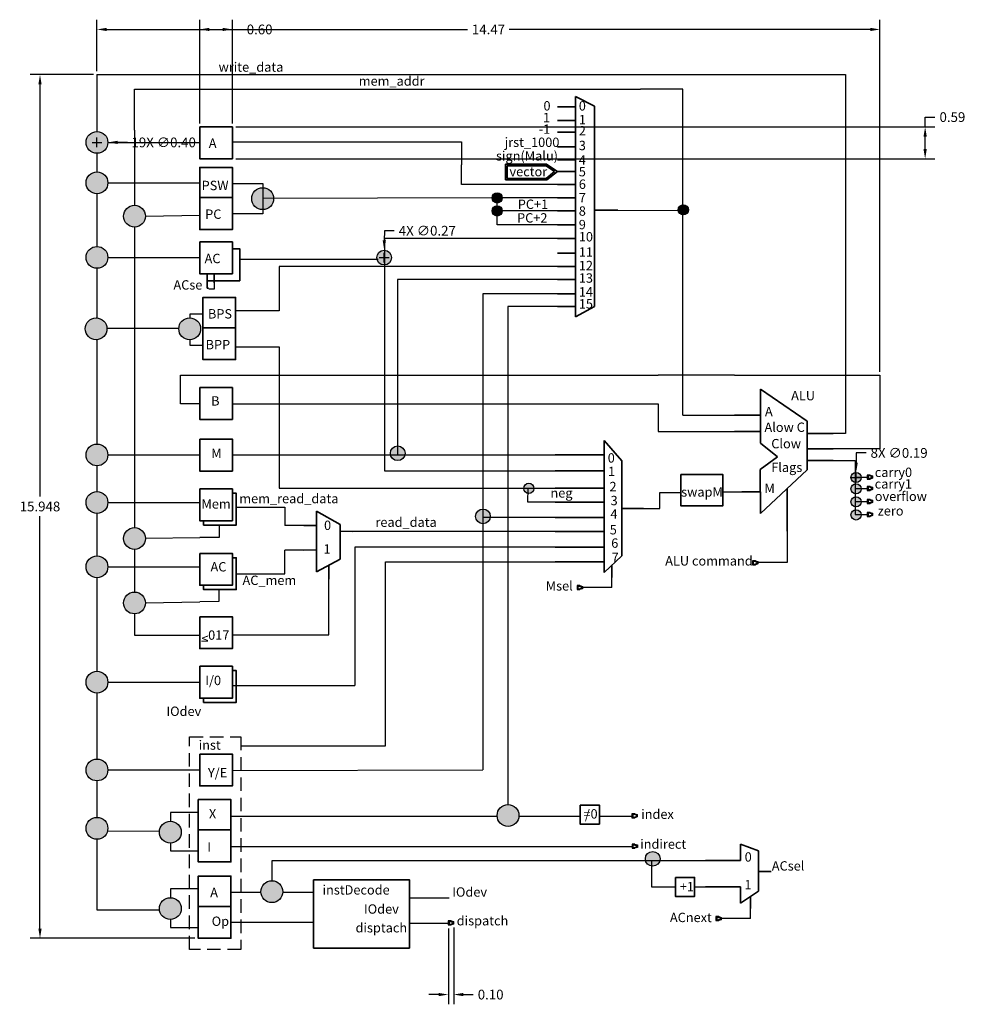
# Model space of a CAD drawing. Units: inches. Extents: x 90.6 to 108.1, y 86.4 to 104.6.
import ezdxf

# ---------------------------------------------------------------- set-up
doc = ezdxf.new("R2010")
doc.units = ezdxf.units.IN
doc.header["$MEASUREMENT"] = 0
doc.linetypes.add('HIDDEN', pattern=[0.375, 0.25, -0.125])
for name, color, linetype, lineweight in [('A-ANNO-DIMS', 2, 'Continuous', 18), ('E-COMP', 1, 'Continuous', 35), ('E-COMP-HIDN', 5, 'HIDDEN', 25), ('E-SYMB', 3, 'Continuous', 25), ('E-TEXT', 4, 'Continuous', 18), ('E-WIRE', 3, 'Continuous', 25)]:
    doc.layers.add(name, color=color, linetype=linetype, lineweight=lineweight)
doc.styles.get("Standard").update_dxf_attribs({"font": 'arial.ttf'})
doc.dimstyles.get("Standard").update_dxf_attribs({"dimtxt": 0.18, "dimasz": 0.18, "dimexe": 0.18, "dimexo": 0.0625, "dimgap": 0.09, "dimtad": 0, "dimtih": 1, "dimtoh": 1, "dimdec": 4, "dimzin": 0, "dimdsep": 46, "dimtxsty": 'Standard', "dimcen": 0.09, "dimadec": 0, "dimazin": 0, "dimtfac": 1, "dimtdec": 4, "dimtofl": 0, "dimtmove": 0, "dimatfit": 3, "dimfxl": 1, "dimtolj": 1, "dimtzin": 0, "dimarcsym": 0})

# ---------------------------------------------------------------- blocks, each defined once
blk = doc.blocks.new('PORT-CONNECTOR')
h = blk.add_hatch(color=256)
h.dxf.hatch_style = 1
h.paths.add_polyline_path([(102.004, 89.371), (101.949, 89.371), (101.949, 89.296), (102.004, 89.296), (102.048, 89.313), (102.048, 89.357), (102.004, 89.371), (102.001, 89.356), (102.033, 89.346), (102.033, 89.323), (102.001, 89.311), (101.965, 89.311), (101.965, 89.356), (102.001, 89.356)])
for p, q in [((101.949, 89.371), (101.949, 89.296)), ((102.004, 89.371), (101.949, 89.371)), ((101.949, 89.296), (102.004, 89.296)), ((101.965, 89.356), (101.965, 89.311)), ((102.001, 89.356), (101.965, 89.356)), ((101.965, 89.311), (102.001, 89.311)), ((102.001, 89.356), (102.033, 89.346)), ((102.033, 89.323), (102.001, 89.311)), ((102.004, 89.371), (102.048, 89.357)), ((102.048, 89.313), (102.004, 89.296)), ((102.033, 89.346), (102.033, 89.323)), ((102.048, 89.357), (102.048, 89.313))]:
    blk.add_line(p, q)
blk = doc.blocks.new('*D2')
at = {"layer": 'A-ANNO-DIMS', "color": 0, "lineweight": -2, "transparency": 16777216}
for p, q in [((92.062, 103.644), (92.062, 104.597)), ((106.531, 98.095), (106.531, 104.597)), ((92.242, 104.417), (98.911, 104.417)), ((106.351, 104.417), (99.682, 104.417))]:
    blk.add_line(p, q, dxfattribs=at)
at = {"layer": 'A-ANNO-DIMS', "color": 0, "transparency": 16777216}
for points in [[(92.242, 104.447), (92.242, 104.387), (92.062, 104.417)], [(106.351, 104.447), (106.351, 104.387), (106.531, 104.417)]]:
    blk.add_solid(points, dxfattribs=at)
at = {"layer": 'Defpoints', "color": 0, "transparency": 16777216}
for p in [(106.531, 104.417), (92.062, 103.582), (106.531, 98.032)]:
    blk.add_point(p, dxfattribs=at)
at = {"layer": 'A-ANNO-DIMS', "color": 0, "transparency": 16777216, "insert": (99.297, 104.417), "char_height": 0.18, "attachment_point": 5}
blk.add_mtext('\\A1;14.47', dxfattribs=at)
blk = doc.blocks.new('*D3')
at = {"layer": 'A-ANNO-DIMS', "color": 0, "lineweight": -2, "transparency": 16777216}
for p, q in [((92, 103.582), (90.829, 103.582)), ((91.009, 103.402), (91.009, 95.79)), ((91.009, 87.814), (91.009, 95.426)), ((93.873, 87.634), (90.829, 87.634))]:
    blk.add_line(p, q, dxfattribs=at)
at = {"layer": 'A-ANNO-DIMS', "color": 0, "transparency": 16777216}
for points in [[(90.979, 103.402), (91.039, 103.402), (91.009, 103.582)], [(90.979, 87.814), (91.039, 87.814), (91.009, 87.634)]]:
    blk.add_solid(points, dxfattribs=at)
at = {"layer": 'Defpoints', "color": 0, "transparency": 16777216}
for p in [(92.062, 103.582), (91.009, 87.634), (93.935, 87.634)]:
    blk.add_point(p, dxfattribs=at)
at = {"layer": 'A-ANNO-DIMS', "color": 0, "transparency": 16777216, "insert": (91.009, 95.608), "char_height": 0.18, "attachment_point": 5}
blk.add_mtext('\\A1;15.948', dxfattribs=at)
blk = doc.blocks.new('*D4')
at = {"layer": 'A-ANNO-DIMS', "color": 0, "lineweight": -2, "transparency": 16777216}
for p, q in [((93.961, 102.68), (93.961, 104.597)), ((94.564, 102.68), (94.564, 104.597)), ((94.141, 104.417), (94.384, 104.417)), ((94.564, 104.417), (94.744, 104.417))]:
    blk.add_line(p, q, dxfattribs=at)
at = {"layer": 'A-ANNO-DIMS', "color": 0, "transparency": 16777216}
for points in [[(94.141, 104.447), (94.141, 104.387), (93.961, 104.417)], [(94.384, 104.447), (94.384, 104.387), (94.564, 104.417)]]:
    blk.add_solid(points, dxfattribs=at)
at = {"layer": 'Defpoints', "color": 0, "transparency": 16777216}
for p in [(94.564, 104.417), (93.961, 102.618), (94.564, 102.618)]:
    blk.add_point(p, dxfattribs=at)
at = {"layer": 'A-ANNO-DIMS', "color": 0, "transparency": 16777216, "insert": (95.068, 104.417), "char_height": 0.18, "attachment_point": 5}
blk.add_mtext('\\A1;0.60', dxfattribs=at)
blk = doc.blocks.new('*D5')
at = {"layer": 'A-ANNO-DIMS', "color": 0, "lineweight": -2, "transparency": 16777216}
for p, q in [((107.366, 102.618), (107.366, 102.798)), ((107.366, 102.798), (107.546, 102.798)), ((94.627, 102.618), (107.546, 102.618)), ((107.366, 102.208), (107.366, 102.438)), ((94.627, 102.028), (107.546, 102.028))]:
    blk.add_line(p, q, dxfattribs=at)
at = {"layer": 'A-ANNO-DIMS', "color": 0, "transparency": 16777216}
for points in [[(107.336, 102.438), (107.396, 102.438), (107.366, 102.618)], [(107.336, 102.208), (107.396, 102.208), (107.366, 102.028)]]:
    blk.add_solid(points, dxfattribs=at)
at = {"layer": 'Defpoints', "color": 0, "transparency": 16777216}
for p in [(94.564, 102.618), (107.366, 102.618), (94.564, 102.028)]:
    blk.add_point(p, dxfattribs=at)
at = {"layer": 'A-ANNO-DIMS', "color": 0, "transparency": 16777216, "insert": (107.87, 102.798), "char_height": 0.18, "attachment_point": 5}
blk.add_mtext('\\A1;0.59', dxfattribs=at)
blk = doc.blocks.new('*D6')
at = {"layer": 'A-ANNO-DIMS', "color": 0, "lineweight": -2, "transparency": 16777216}
for p, q in [((98.654, 87.835), (98.654, 86.415)), ((98.555, 87.818), (98.555, 86.415)), ((98.375, 86.595), (98.195, 86.595)), ((98.834, 86.595), (99.014, 86.595))]:
    blk.add_line(p, q, dxfattribs=at)
at = {"layer": 'A-ANNO-DIMS', "color": 0, "transparency": 16777216}
for points in [[(98.375, 86.625), (98.375, 86.565), (98.555, 86.595)], [(98.834, 86.625), (98.834, 86.565), (98.654, 86.595)]]:
    blk.add_solid(points, dxfattribs=at)
at = {"layer": 'Defpoints', "color": 0, "transparency": 16777216}
for p in [(98.555, 87.88), (98.654, 87.897), (98.654, 86.595)]:
    blk.add_point(p, dxfattribs=at)
at = {"layer": 'A-ANNO-DIMS', "color": 0, "transparency": 16777216, "insert": (99.337, 86.595), "char_height": 0.18, "attachment_point": 5}
blk.add_mtext('\\A1;0.10', dxfattribs=at)
blk = doc.blocks.new('*D7')
at = {"layer": 'A-ANNO-DIMS', "color": 0, "lineweight": -2, "transparency": 16777216}
for p, q in [((92.062, 102.241), (92.062, 102.421)), ((91.972, 102.331), (92.152, 102.331)), ((92.624, 102.331), (92.444, 102.331))]:
    blk.add_line(p, q, dxfattribs=at)
at = {"layer": 'A-ANNO-DIMS', "color": 0, "transparency": 16777216}
blk.add_solid([(92.444, 102.361), (92.444, 102.301), (92.264, 102.331)], dxfattribs=at)
at = {"layer": 'Defpoints', "color": 0, "transparency": 16777216}
for p in [(91.86, 102.331), (92.264, 102.331)]:
    blk.add_point(p, dxfattribs=at)
at = {"layer": 'A-ANNO-DIMS', "color": 0, "transparency": 16777216, "insert": (93.295, 102.331), "char_height": 0.18, "attachment_point": 5}
blk.add_mtext('\\A1;19X ∅0.40', dxfattribs=at)
blk = doc.blocks.new('*D8')
at = {"layer": 'A-ANNO-DIMS', "color": 0, "lineweight": -2, "transparency": 16777216}
for p, q in [((97.374, 100.7), (97.372, 100.52)), ((97.554, 100.7), (97.374, 100.7)), ((97.279, 100.204), (97.459, 100.204)), ((97.369, 100.114), (97.369, 100.294))]:
    blk.add_line(p, q, dxfattribs=at)
at = {"layer": 'A-ANNO-DIMS', "color": 0, "transparency": 16777216}
blk.add_solid([(97.342, 100.521), (97.402, 100.52), (97.37, 100.34)], dxfattribs=at)
at = {"layer": 'Defpoints', "color": 0, "transparency": 16777216}
for p in [(97.37, 100.34), (97.367, 100.068)]:
    blk.add_point(p, dxfattribs=at)
at = {"layer": 'A-ANNO-DIMS', "color": 0, "transparency": 16777216, "insert": (98.167, 100.7), "char_height": 0.18, "attachment_point": 5}
blk.add_mtext('\\A1;4X ∅0.27', dxfattribs=at)
blk = doc.blocks.new('*D9')
at = {"layer": 'A-ANNO-DIMS', "color": 0, "lineweight": -2, "transparency": 16777216}
for p, q in [((106.094, 96.597), (106.092, 96.417)), ((106.274, 96.597), (106.094, 96.597)), ((106.089, 96.053), (106.089, 96.233)), ((105.999, 96.143), (106.179, 96.143))]:
    blk.add_line(p, q, dxfattribs=at)
at = {"layer": 'A-ANNO-DIMS', "color": 0, "transparency": 16777216}
blk.add_solid([(106.062, 96.417), (106.122, 96.417), (106.09, 96.237)], dxfattribs=at)
at = {"layer": 'Defpoints', "color": 0, "transparency": 16777216}
for p in [(106.09, 96.237), (106.088, 96.049)]:
    blk.add_point(p, dxfattribs=at)
at = {"layer": 'A-ANNO-DIMS', "color": 0, "transparency": 16777216, "insert": (106.885, 96.597), "char_height": 0.18, "attachment_point": 5}
blk.add_mtext('\\A1;8X ∅0.19', dxfattribs=at)

msp = doc.modelspace()

# ---------------------------------------------------------------- hatches: boundary and pattern name
at = {"layer": 'E-COMP'}
h = msp.add_hatch(color=256, dxfattribs=at)
h.dxf.hatch_style = 1
h.paths.add_polyline_path([(99.6422, 101.9276), (99.6122, 101.9276), (99.6122, 101.8976), (99.6122, 101.6671), (99.6122, 101.6371), (99.6422, 101.6371), (99.6422, 101.6671)])
h.paths.add_polyline_path([(100.3621, 101.6671), (99.6422, 101.6671), (99.6422, 101.6371), (100.3621, 101.6371)])
h.paths.add_polyline_path([(100.3621, 101.9276), (99.6422, 101.9276), (99.6422, 101.8976), (100.3621, 101.8976)])
h.paths.add_polyline_path([(100.3713, 101.9276), (100.3621, 101.9276), (100.3621, 101.8976), (100.5192, 101.7913), (100.5676, 101.7913), (100.57, 101.7932)])
h.paths.add_polyline_path([(100.5676, 101.7913), (100.5192, 101.7913), (100.3621, 101.6671), (100.3621, 101.6371), (100.3726, 101.6371)])
at = {"layer": 'E-SYMB'}
h = msp.add_hatch(color=256, dxfattribs=at)
h.dxf.hatch_style = 1
h.paths.add_polyline_path([(106.0735, 96.2356, 0.366956), (105.9948, 96.1428, 0.366956), (106.0735, 96.05)])
h.paths.add_polyline_path([(106.0735, 96.2356), (106.0735, 96.1478), (106.1828, 96.1478, 0.4472138)])
h.paths.add_polyline_path([(106.183, 96.1428, 0.0131646), (106.1828, 96.1478), (106.0735, 96.1478), (106.0735, 96.05, 0.4631049)])
h.paths.add_polyline_path([(106.0735, 96.0262), (106.0735, 95.9383), (106.1828, 95.9383, 0.4472138)])
h.paths.add_polyline_path([(106.183, 95.9334, 0.0131646), (106.1828, 95.9383), (106.0735, 95.9383), (106.0735, 95.8405, 0.4631049)])
h.paths.add_polyline_path([(106.0735, 95.9383), (106.0735, 96.0262, 0.366956), (105.9948, 95.9334, 0.366956), (106.0735, 95.8405)])
h.paths.add_polyline_path([(106.0735, 95.7855, 0.366956), (105.9948, 95.6927, 0.366956), (106.0735, 95.5999)])
h.paths.add_polyline_path([(106.0735, 95.7855), (106.0735, 95.6976), (106.1828, 95.6976, 0.4472138)])
h.paths.add_polyline_path([(106.183, 95.6927, 0.0131646), (106.1828, 95.6976), (106.0735, 95.6976), (106.0735, 95.5999, 0.4631049)])
h.paths.add_polyline_path([(106.0735, 95.5448, 0.366956), (105.9948, 95.452, 1), (106.183, 95.452, 0.0131646), (106.1828, 95.4569), (106.0735, 95.4569)])
h.paths.add_polyline_path([(106.0735, 95.5448), (106.0735, 95.4569), (106.1828, 95.4569, 0.4472138)])
h.paths.add_polyline_path([(100.138, 95.9425, 0.0131646), (100.1379, 95.9475), (100.0286, 95.9475), (100.0266, 95.85, 0.4696785)])
h.paths.add_polyline_path([(100.0286, 95.9475), (99.95, 95.9475, 0.0131646), (99.9499, 95.9425, 0.3608418), (100.0266, 95.85)])
h.paths.add_polyline_path([(99.95, 95.9475), (100.0286, 95.9475), (100.1379, 95.9475, 0.9486838)])
h.paths.add_polyline_path([(99.4565, 89.9015, 1), (99.8599, 89.9015, 1)])
h.paths.add_polyline_path([(95.0927, 88.495, 1), (95.4961, 88.495, 1)])
h.paths.add_polyline_path([(93.2164, 88.1826, 1), (93.6198, 88.1826, 1)])
h.paths.add_polyline_path([(93.6198, 89.5947, 1), (93.2164, 89.5947, 1)])
h.paths.add_polyline_path([(92.2638, 89.6647, 1), (91.8604, 89.6647, 1)])
h.paths.add_polyline_path([(91.8604, 90.7425, 1), (92.2638, 90.7425, 1)])
h.paths.add_polyline_path([(92.2638, 92.3637, 1), (91.8604, 92.3637, 1)])
h.paths.add_polyline_path([(92.9584, 93.8266, 1), (92.555, 93.8266, 1)])
h.paths.add_polyline_path([(92.2638, 94.4942, 1), (91.8604, 94.4942, 1)])
h.paths.add_polyline_path([(92.555, 95.0169, 1), (92.9584, 95.0169, 1)])
h.paths.add_polyline_path([(91.8604, 95.6825, 1), (92.2638, 95.6825, 1)])
h.paths.add_polyline_path([(91.8604, 96.5597, 1), (92.2638, 96.5597, 1)])
h.paths.add_polyline_path([(91.8437, 98.8894, 1), (92.247, 98.8894, 1)])
h.paths.add_polyline_path([(93.5739, 98.8894, 1), (93.9773, 98.8894, 1)])
h.paths.add_polyline_path([(91.8604, 100.2075, 1), (92.2638, 100.2075, 1)])
h.paths.add_polyline_path([(92.555, 100.9676, 1), (92.9584, 100.9676, 1)])
h.paths.add_polyline_path([(91.8604, 101.5837, 1), (92.2638, 101.5837, 1)])
h.paths.add_polyline_path([(92.2638, 102.3309, 1), (91.8604, 102.3309, 1)])
h = msp.add_hatch(color=256, dxfattribs=at)
h.dxf.hatch_style = 1
h.paths.add_polyline_path([(95.1242, 101.09, 0.4142136), (95.3259, 101.2917, 0.4142136), (95.1242, 101.4934)])
h.paths.add_polyline_path([(94.9225, 101.2917, 0.4142136), (95.1242, 101.09), (95.1242, 101.4934, 0.4142136)])
h = msp.add_hatch(color=256, dxfattribs=at)
h.dxf.hatch_style = 1
h.paths.add_polyline_path([(99.5508, 101.3059, 1), (99.3627, 101.3059, 1)])
h = msp.add_hatch(color=256, dxfattribs=at)
h.dxf.hatch_style = 1
h.paths.add_polyline_path([(99.4567, 101.1597, 0.4144064), (99.3626, 101.0656, 0.4143029), (99.4567, 100.9715)])
h.paths.add_polyline_path([(99.5507, 101.0656), (99.4567, 101.0656), (99.4567, 100.9715, 0.4141242)])
h.paths.add_polyline_path([(99.4567, 101.1597), (99.4567, 101.0656), (99.5507, 101.0656, 0.4140208)])
h = msp.add_hatch(color=256, dxfattribs=at)
h.dxf.hatch_style = 1
h.paths.add_polyline_path([(102.8877, 101.1789, 0.3829883), (102.8038, 101.0853, 0.3829883), (102.8877, 100.9918)])
h.paths.add_polyline_path([(102.8877, 101.1789), (102.8877, 100.9918, 0.4461438), (102.9919, 101.0853, 0.4461438)])
h = msp.add_hatch(color=256, dxfattribs=at)
h.dxf.hatch_style = 1
h.paths.add_polyline_path([(97.5049, 100.2039, 1), (97.2324, 100.2039, 1)])
h = msp.add_hatch(color=256, dxfattribs=at)
h.dxf.hatch_style = 1
h.paths.add_polyline_path([(97.7557, 96.5908, 1), (97.4832, 96.5908, 1)])
h = msp.add_hatch(color=256, dxfattribs=at)
h.dxf.hatch_style = 1
h.paths.add_polyline_path([(99.3309, 95.4246, 1), (99.0583, 95.4246, 1)])
h = msp.add_hatch(color=256, dxfattribs=at)
h.dxf.hatch_style = 1
h.paths.add_polyline_path([(102.4683, 89.1009, 1), (102.1957, 89.1009, 1)])

# ---------------------------------------------------------------- linework, layer by layer
at = {"layer": 'E-COMP'}
for p, q in [((100.9022, 103.1788), (100.9022, 99.1114)), ((101.2566, 102.9982), (100.9022, 103.1788)), ((100.9022, 102.9879), (100.57, 102.9879)), ((101.2566, 102.8182), (101.2566, 102.9982)), ((100.9022, 102.7363), (100.57, 102.7363)), ((101.2566, 102.8182), (101.2566, 99.2988)), ((100.9022, 102.5213), (100.57, 102.5213)), ((100.9022, 102.2463), (100.57, 102.2463)), ((100.9022, 102.0082), (100.57, 102.0082)), ((99.6122, 101.9276), (100.3621, 101.9276)), ((99.6122, 101.8976), (99.6122, 101.9276)), ((99.6122, 101.8976), (99.6122, 101.6671)), ((99.6422, 101.8976), (100.3621, 101.8976)), ((99.6422, 101.8976), (99.6422, 101.6671)), ((99.6422, 101.8976), (99.6422, 101.6671)), ((100.2827, 101.9845), (100.2827, 101.9845)), ((100.3621, 101.9276), (100.3713, 101.9276)), ((100.5192, 101.7913), (100.3621, 101.8976)), ((100.57, 101.7932), (100.3713, 101.9276)), ((99.6122, 101.6671), (99.6122, 101.6371)), ((99.6122, 101.6371), (100.3621, 101.6371)), ((99.6422, 101.6671), (100.3621, 101.6671)), ((100.3621, 101.6671), (100.5192, 101.7913)), ((100.3621, 101.6371), (100.3726, 101.6371)), ((100.3726, 101.6371), (100.57, 101.7932)), ((100.9022, 101.7932), (100.57, 101.7932)), ((100.9022, 101.5554), (100.57, 101.5554)), ((94.564, 101.3106), (93.9606, 101.3106)), ((100.9022, 101.308), (100.57, 101.308)), ((100.9022, 101.0656), (100.57, 101.0656)), ((101.2566, 101.0774), (101.6846, 101.0774)), ((100.9022, 100.8089), (100.57, 100.8089)), ((100.9022, 100.5569), (100.57, 100.5569)), ((100.9022, 100.287), (100.57, 100.287)), ((100.9022, 100.0395), (100.57, 100.0395)), ((94.2271, 99.9048), (94.2271, 99.7376)), ((94.0975, 99.7767), (94.0975, 99.6376)), ((94.0975, 99.6376), (94.1227, 99.6376)), ((100.9022, 99.8017), (100.57, 99.8017)), ((100.9022, 99.5359), (100.57, 99.5359)), ((100.9022, 99.3027), (100.57, 99.3027)), ((101.2566, 99.2988), (100.9022, 99.1114)), ((94.6224, 98.9092), (94.019, 98.9092)), ((104.3231, 96.7766), (104.3231, 97.7766)), ((104.3231, 97.7766), (105.1867, 97.1862)), ((103.8454, 97.2961), (104.3231, 97.2961)), ((105.1867, 97.1862), (105.1867, 96.2862)), ((103.8454, 96.9943), (104.3231, 96.9943)), ((105.6692, 96.9538), (105.1867, 96.9538)), ((101.4328, 96.8253), (101.4328, 94.3862)), ((101.4328, 96.8253), (101.763, 96.4499)), ((104.3231, 96.7766), (104.6361, 96.5275)), ((100.5301, 96.5597), (101.4328, 96.5597)), ((105.6692, 96.6702), (105.1867, 96.6702)), ((101.763, 96.4499), (101.763, 94.6945)), ((104.6361, 96.5275), (104.3151, 96.2888)), ((105.6692, 96.456), (105.1867, 96.456)), ((100.5301, 96.2671), (101.4328, 96.2671)), ((104.3151, 96.2888), (104.3231, 95.4807)), ((104.3231, 95.4807), (105.1867, 96.2862)), ((100.5301, 95.9475), (101.4328, 95.9475)), ((103.9768, 95.8772), (104.3192, 95.8772)), ((104.8174, 95.9418), (104.8174, 95.1508)), ((100.5301, 95.6867), (101.4328, 95.6867)), ((96.1184, 95.5225), (96.1184, 94.399)), ((96.1184, 95.5225), (96.5539, 95.2768)), ((101.763, 95.5677), (102.163, 95.5677)), ((96.5539, 95.2768), (96.5539, 94.637)), ((100.5301, 95.4044), (101.4328, 95.4044)), ((95.8832, 95.2564), (96.1184, 95.2575)), ((96.7771, 95.1479), (96.5539, 95.1513)), ((100.5301, 95.1479), (101.4328, 95.1479)), ((95.8832, 94.8036), (96.1184, 94.8066)), ((100.5301, 94.8571), (101.4328, 94.8571)), ((96.1184, 94.399), (96.5581, 94.637)), ((100.5301, 94.5834), (101.4328, 94.5834)), ((101.4328, 94.3862), (101.763, 94.6945)), ((96.3453, 94.5218), (96.3453, 94.2656)), ((101.5754, 94.2936), (101.5754, 94.5193)), ((94.5385, 89.635), (93.9351, 89.635)), ((103.9561, 89.0697), (103.9561, 89.3697)), ((104.2877, 89.2495), (103.9561, 89.3697)), ((104.2877, 88.5062), (104.2877, 89.2495)), ((103.3092, 89.0697), (103.9561, 89.0697)), ((104.2877, 88.8659), (104.5204, 88.8659)), ((103.3092, 88.5826), (103.9561, 88.5826)), ((103.9561, 88.5826), (103.9561, 88.2826)), ((103.9561, 88.2826), (104.2877, 88.5062)), ((104.1412, 88.1817), (104.1412, 88.4074)), ((94.5385, 88.2228), (93.9351, 88.2228))]:
    msp.add_line(p, q, dxfattribs=at)
for points in [[(93.9606, 102.6176), (94.564, 102.6176), (94.564, 102.0283), (93.9606, 102.0283)], [(93.9606, 100.4941), (94.564, 100.4941), (94.564, 99.9048), (93.9606, 99.9048)], [(93.9606, 100.4941), (94.564, 100.4941), (94.564, 99.9048), (93.9606, 99.9048)], [(93.9606, 97.8034), (94.564, 97.8034), (94.564, 97.2141), (93.9606, 97.2141)], [(93.9606, 96.851), (94.564, 96.851), (94.564, 96.2617), (93.9606, 96.2617)], [(102.8515, 96.1981), (103.6272, 96.1996), (103.6272, 95.6197), (102.8515, 95.6183)], [(93.9606, 95.9322), (94.564, 95.9322), (94.564, 95.3429), (93.9606, 95.3429)], [(93.9606, 94.7417), (94.564, 94.7417), (94.564, 94.1525), (93.9606, 94.1525)], [(93.9606, 93.573), (94.564, 93.573), (94.564, 92.9837), (93.9606, 92.9837)], [(93.9606, 92.6569), (94.564, 92.6569), (94.564, 92.0676), (93.9606, 92.0676)], [(93.9606, 91.0357), (94.564, 91.0357), (94.564, 90.4464), (93.9606, 90.4464)], [(100.9907, 90.0948), (101.3458, 90.0948), (101.3458, 89.7435), (100.9907, 89.7435)], [(102.7507, 88.7586), (103.1057, 88.7586), (103.1057, 88.4073), (102.7507, 88.4073)], [(96.0648, 88.7163), (97.8365, 88.7163), (97.8365, 87.4518), (96.0648, 87.4518)]]:
    msp.add_lwpolyline(points, close=True, dxfattribs=at)
for points in [[(93.9606, 101.2811), (93.9606, 101.8704), (94.564, 101.8704), (94.564, 101.2811)], [(94.564, 101.3106), (94.564, 100.7213), (93.9606, 100.7213), (93.9606, 101.3106)], [(94.564, 100.366), (94.7009, 100.366), (94.7009, 99.7767), (94.0975, 99.7767), (94.0975, 99.9048)], [(94.019, 98.8797), (94.019, 99.469), (94.6224, 99.469), (94.6224, 98.8797)], [(94.6224, 98.9092), (94.6224, 98.3199), (94.019, 98.3199), (94.019, 98.9092)], [(94.564, 95.8529), (94.6344, 95.8529), (94.6344, 95.2637), (94.031, 95.2637), (94.031, 95.3429)], [(94.564, 94.6625), (94.6344, 94.6625), (94.6344, 94.0732), (94.031, 94.0732), (94.031, 94.1525)], [(94.564, 92.5776), (94.6344, 92.5776), (94.6344, 91.9884), (94.031, 91.9884), (94.031, 92.0676)], [(93.9351, 89.6055), (93.9351, 90.1948), (94.5385, 90.1948), (94.5385, 89.6055)], [(94.5385, 89.635), (94.5385, 89.0457), (93.9351, 89.0457), (93.9351, 89.635)], [(93.9351, 88.1934), (93.9351, 88.7827), (94.5385, 88.7827), (94.5385, 88.1934)], [(94.5385, 88.2228), (94.5385, 87.6336), (93.9351, 87.6336), (93.9351, 88.2228)]]:
    msp.add_lwpolyline(points, dxfattribs=at)
at = {"layer": 'E-COMP-HIDN'}
msp.add_lwpolyline([(93.7723, 91.3553), (94.7228, 91.3553), (94.7228, 87.4301), (93.7723, 87.4301)], close=True, dxfattribs=at)
at = {"layer": 'E-SYMB'}
for centre, radius in [((92.0621, 102.3309), 0.2017), ((92.0621, 101.5837), 0.2017), ((95.1242, 101.2917), 0.2017), ((99.4567, 101.3059), 0.0941), ((92.7567, 100.9676), 0.2017), ((99.4567, 101.0656), 0.0941), ((102.8978, 101.0853), 0.0941), ((92.0621, 100.2075), 0.2017), ((97.3687, 100.2039), 0.1363), ((92.0454, 98.8894), 0.2017), ((93.7756, 98.8894), 0.2017), ((92.0621, 96.5597), 0.2017), ((97.6195, 96.5908), 0.1363), ((106.0889, 96.1428), 0.0941), ((100.0439, 95.9425), 0.0941), ((106.0889, 95.9334), 0.0941), ((92.0621, 95.6825), 0.2017), ((106.0889, 95.6927), 0.0941), ((99.1946, 95.4246), 0.1363), ((106.0889, 95.452), 0.0941), ((92.7567, 95.0169), 0.2017), ((92.0621, 94.4942), 0.2017), ((92.7567, 93.8266), 0.2017), ((92.0621, 92.3637), 0.2017), ((92.0621, 90.7425), 0.2017), ((99.6582, 89.9015), 0.2017), ((92.0621, 89.6647), 0.2017), ((93.4181, 89.5947), 0.2017), ((102.332, 89.1009), 0.1363), ((95.2944, 88.495), 0.2017), ((93.4181, 88.1826), 0.2017)]:
    msp.add_circle(centre, radius, dxfattribs=at)
at = {"layer": 'E-WIRE'}
for p, q in [((92.0621, 103.5818), (92.0621, 102.5326)), ((92.0621, 103.5818), (102.1048, 103.5818)), ((102.1048, 103.5818), (105.8923, 103.5818)), ((105.8923, 103.5818), (105.8923, 96.9538)), ((92.7567, 102.5585), (92.7567, 103.312)), ((92.7567, 103.312), (102.1048, 103.312)), ((102.8877, 103.312), (102.1048, 103.312)), ((102.8877, 97.2961), (102.8877, 103.312)), ((92.7567, 102.5585), (92.7567, 101.1693)), ((92.2638, 102.3309), (93.9606, 102.3309)), ((94.564, 102.3419), (98.7972, 102.3419)), ((98.7972, 102.3419), (98.7972, 101.9162)), ((92.0621, 102.1293), (92.0621, 101.7854)), ((98.7972, 101.5554), (98.7972, 101.9162)), ((92.2638, 101.5837), (93.9606, 101.5837)), ((94.564, 101.571), (95.1242, 101.571)), ((95.1242, 101.571), (95.1242, 101.0092)), ((100.57, 101.5554), (98.7972, 101.5554)), ((92.0621, 101.3821), (92.0621, 100.4092)), ((99.3627, 101.3057), (95.1242, 101.2976)), ((100.57, 101.308), (99.5508, 101.3061)), ((99.4567, 100.8089), (99.4567, 101.2118)), ((92.9584, 100.9709), (93.9606, 100.9869)), ((95.1242, 101.0092), (94.564, 101.0092)), ((100.57, 101.0656), (99.4567, 101.0656)), ((101.6846, 101.0774), (102.8045, 101.0736)), ((92.7567, 100.7659), (92.7567, 96.9192)), ((100.57, 100.8089), (99.4567, 100.8089)), ((100.57, 100.5569), (97.375, 100.5569)), ((97.375, 100.5569), (97.375, 98.8719)), ((92.2638, 100.2075), (93.9606, 100.2075)), ((92.0621, 100.0058), (92.0621, 99.0904)), ((94.7009, 100.1728), (97.2563, 100.1728)), ((100.57, 100.0395), (95.431, 100.0395)), ((95.431, 100.0395), (95.431, 99.2229)), ((94.2271, 99.7376), (94.2271, 99.6199)), ((100.57, 99.8017), (97.6168, 99.8017)), ((97.6168, 99.8017), (97.6168, 98.8221)), ((94.2271, 99.6199), (94.1308, 99.6199)), ((100.57, 99.5359), (99.1913, 99.5359)), ((99.1913, 99.5359), (99.1913, 98.591)), ((100.57, 99.3027), (99.6538, 99.3027)), ((99.6538, 99.3027), (99.6538, 98.5732)), ((94.019, 99.161), (93.7756, 99.161)), ((93.7756, 99.161), (93.7756, 99.0911)), ((95.431, 99.2229), (94.6224, 99.2234)), ((93.574, 98.8942), (92.247, 98.8942)), ((97.375, 98.8719), (97.375, 96.2671)), ((97.6168, 98.8221), (97.6168, 96.5597)), ((92.0621, 98.6884), (92.0621, 96.7614)), ((93.7756, 98.6877), (93.7756, 98.5867)), ((93.7756, 98.5867), (94.019, 98.5837)), ((94.6224, 98.5567), (95.431, 98.5567)), ((95.431, 98.5567), (95.431, 98.5567)), ((95.431, 98.5567), (95.431, 95.9475)), ((99.1913, 98.591), (99.1913, 90.7436)), ((99.6538, 98.5732), (99.6538, 90.1032)), ((93.6042, 97.5048), (93.6042, 98.0325)), ((93.6042, 98.0325), (102.4312, 98.0325)), ((103.8454, 98.0325), (102.4312, 98.0325)), ((103.8454, 98.0325), (106.531, 98.0325)), ((106.531, 98.0325), (106.531, 96.6702)), ((93.9606, 97.5048), (93.6042, 97.5048)), ((94.564, 97.5048), (102.4312, 97.5048)), ((102.4312, 97.5048), (102.4312, 96.9943)), ((102.8877, 97.2961), (103.8454, 97.2961)), ((92.7567, 96.9192), (92.7567, 95.2186)), ((102.4312, 96.9943), (103.8454, 96.9943)), ((105.8923, 96.9538), (105.6692, 96.9538)), ((92.2638, 96.5597), (93.9606, 96.5597)), ((94.564, 96.5597), (100.5301, 96.5597)), ((106.531, 96.6702), (105.6692, 96.6702)), ((105.6692, 96.456), (106.0735, 96.456)), ((106.0735, 96.456), (106.0735, 95.4569)), ((92.0621, 96.358), (92.0621, 95.8842)), ((97.375, 96.2671), (100.5301, 96.2671)), ((106.0735, 96.1478), (106.2965, 96.1478)), ((95.431, 95.9475), (98.9728, 95.9475)), ((98.9728, 95.9475), (100.5301, 95.9475)), ((100.0232, 95.6867), (100.0286, 95.9475)), ((102.463, 95.5677), (102.463, 95.8677)), ((102.463, 95.8677), (102.8515, 95.8677)), ((103.6272, 95.8772), (103.9768, 95.8772)), ((106.0735, 95.9383), (106.2965, 95.9383)), ((92.2638, 95.6825), (93.9606, 95.6825)), ((100.5301, 95.6867), (100.0232, 95.6867)), ((106.0735, 95.6976), (106.2965, 95.6976)), ((92.0621, 95.4808), (92.0621, 94.6959)), ((94.6344, 95.5973), (95.5364, 95.5973)), ((95.5364, 95.5973), (95.5364, 95.2564)), ((102.163, 95.5677), (102.463, 95.5677)), ((106.0735, 95.4569), (106.2965, 95.4569)), ((100.5301, 95.4044), (99.1913, 95.4044)), ((94.3232, 95.2637), (94.3232, 95.0362)), ((95.8832, 95.2564), (95.5364, 95.2564)), ((100.5301, 95.1479), (96.7771, 95.1479)), ((104.8174, 95.1508), (104.8174, 94.5705)), ((92.9584, 95.0201), (93.9606, 95.0362)), ((94.3232, 95.0362), (93.9606, 95.0362)), ((92.7567, 94.8152), (92.7567, 94.0283)), ((95.8832, 94.8036), (95.5364, 94.8036)), ((95.5364, 94.3621), (95.5364, 94.8036)), ((100.5301, 94.8571), (96.8296, 94.8571)), ((96.8296, 94.8571), (96.8296, 92.2993)), ((97.3938, 91.1859), (97.3938, 94.5834)), ((97.3938, 94.5834), (100.5301, 94.5834)), ((104.8174, 94.5705), (104.274, 94.5705)), ((92.2638, 94.4942), (93.9606, 94.4942)), ((92.0621, 94.2925), (92.0621, 92.5654)), ((94.6344, 94.3621), (95.5364, 94.3621)), ((96.3453, 93.238), (96.3453, 94.2656)), ((101.5754, 94.1125), (101.5754, 94.2936)), ((94.3112, 94.0732), (94.3112, 93.8516)), ((101.5754, 94.1125), (101.032, 94.1125)), ((92.9584, 93.8299), (93.9606, 93.8459)), ((94.3112, 93.8516), (93.9606, 93.8459)), ((92.7567, 93.625), (92.7567, 93.2293)), ((92.7567, 93.2293), (93.9606, 93.2293)), ((94.564, 93.238), (96.3453, 93.238)), ((92.2638, 92.3637), (93.9606, 92.3637)), ((94.564, 92.2993), (96.8296, 92.2993)), ((92.0621, 92.162), (92.0621, 90.9441)), ((94.7228, 91.1859), (97.3938, 91.1859)), ((92.2638, 90.7425), (93.9606, 90.7425)), ((94.564, 90.7348), (99.1913, 90.7436)), ((92.0621, 90.5408), (92.0621, 89.8663)), ((93.9351, 89.9599), (93.4181, 89.9599)), ((93.4181, 89.9599), (93.4181, 89.7964)), ((94.5385, 89.8921), (99.4568, 89.8921)), ((99.8597, 89.8921), (100.9907, 89.8921)), ((101.3458, 89.8921), (101.9478, 89.8921)), ((92.0621, 89.463), (92.0621, 88.1586)), ((92.2582, 89.6175), (93.2173, 89.6135)), ((93.4181, 89.3931), (93.4181, 89.2484)), ((94.5385, 89.3303), (101.0055, 89.3303)), ((101.0055, 89.3303), (101.9495, 89.3303)), ((93.4181, 89.2484), (93.9351, 89.2484)), ((95.2969, 88.6967), (95.2969, 89.0697)), ((95.2969, 89.0697), (103.3092, 89.0697)), ((102.3069, 89.0697), (102.3069, 88.5826)), ((93.9351, 88.5477), (93.4181, 88.5477)), ((93.4181, 88.5477), (93.4181, 88.3843)), ((102.3069, 88.5826), (102.7485, 88.5826)), ((102.7485, 88.5826), (102.7507, 88.5826)), ((103.1057, 88.5826), (103.3092, 88.5826)), ((92.0621, 88.5082), (92.0621, 88.1586)), ((94.5385, 88.4855), (95.0929, 88.4855)), ((95.4958, 88.4855), (96.0648, 88.4855)), ((97.8365, 88.3806), (98.5681, 88.3806)), ((104.1412, 88.0007), (104.1412, 88.1817)), ((92.0621, 88.1586), (93.2179, 88.1586)), ((104.1412, 88.0007), (103.5978, 88.0007)), ((93.4181, 87.9809), (93.4181, 87.8363)), ((93.4181, 87.8363), (93.9351, 87.8363)), ((94.5385, 87.9303), (96.0648, 87.9303)), ((97.8365, 87.9144), (98.5681, 87.9144))]:
    msp.add_line(p, q, dxfattribs=at)

# ---------------------------------------------------------------- block references
at = {"layer": 'E-SYMB'}
for p in [(4.347, 6.8175), (4.347, 6.608), (4.347, 6.3674), (4.347, 6.1267), (2.2257, 5.2339), (-1.0163, 4.776), (-0.0017, 0.5618), (0, 0), (1.5495, -1.3359), (-3.3947, -1.4158)]:
    msp.add_blockref('PORT-CONNECTOR', p, dxfattribs=at)

# ---------------------------------------------------------------- texts
at = {"layer": 'E-TEXT'}
for s, height, p in [('write_data', 0.17282, (94.3095, 103.6362)), ('mem_addr', 0.17282, (96.8998, 103.3778)), ('0', 0.1728, (100.3131, 102.9205)), ('0', 0.1728, (100.9659, 102.9186)), ('1', 0.1728, (100.3035, 102.7034)), ('1', 0.1728, (100.9659, 102.6643)), ('-1', 0.17282, (100.2257, 102.4894)), ('2', 0.1728, (100.9659, 102.4594)), ('A', 0.1728, (94.1281, 102.2302)), ('jrst_1000', 0.17282, (99.5963, 102.2468)), ('sign(Malu)', 0.17282, (99.4358, 101.9946)), ('3', 0.1728, (100.9659, 102.1871)), ('4', 0.1728, (100.9659, 101.9207)), ('vector', 0.17282, (99.6851, 101.7052)), ('5', 0.1728, (100.9659, 101.7039)), ('6', 0.1728, (100.9659, 101.473)), ('PSW', 0.17282, (93.996, 101.449)), ('PC+1', 0.17282, (99.8384, 101.1021)), ('7', 0.1728, (100.9659, 101.2219)), ('PC', 0.17282, (94.0622, 100.9195)), ('8', 0.1728, (100.9659, 100.9772)), ('PC+2', 0.17282, (99.8255, 100.8509)), ('9', 0.1728, (100.9659, 100.7269)), ('10', 0.17282, (100.9659, 100.5019)), ('11', 0.17282, (100.9659, 100.2199)), ('AC', 0.17282, (94.0505, 100.1006)), ('12', 0.17282, (100.9659, 99.9709)), ('13', 0.17282, (100.9659, 99.7398)), ('ACse', 0.17282, (93.4751, 99.6132)), ('14', 0.17282, (100.9659, 99.485)), ('15', 0.17282, (100.9659, 99.2635)), ('BPS', 0.17282, (94.1129, 99.079)), ('BPP', 0.17282, (94.07, 98.5106)), ('B', 0.1728, (94.1721, 97.471)), ('ALU', 0.17282, (104.8899, 97.5683)), ('A', 0.1728, (104.4056, 97.2749)), ('Alow C', 0.17282, (104.397, 96.9849)), ('Clow', 0.17282, (104.5226, 96.6818)), ('M', 0.1728, (94.1733, 96.5053)), ('0', 0.1728, (101.5002, 96.4179)), ('Flags', 0.17282, (104.5226, 96.2445)), ('1', 0.1728, (101.5062, 96.1685)), ('carry0', 0.17282, (106.4355, 96.1526)), ('2', 0.1728, (101.5334, 95.8896)), ('M', 0.1728, (104.397, 95.8549)), ('carry1', 0.17282, (106.4337, 95.9394)), ('mem_read_data', 0.17282, (94.692, 95.6675)), ('neg', 0.17282, (100.4424, 95.7713)), ('swapM', 0.17282, (102.8574, 95.7893)), ('overflow', 0.17282, (106.4355, 95.7085)), ('Mem', 0.17282, (93.9927, 95.5688)), ('3', 0.1728, (101.553, 95.6309)), ('4', 0.1728, (101.5499, 95.3826)), ('zero', 0.17282, (106.4898, 95.4412)), ('0', 0.1728, (96.2584, 95.1738)), ('read_data', 0.17282, (97.2074, 95.2314)), ('5', 0.1728, (101.5379, 95.0922)), ('1', 0.1728, (96.2484, 94.7371)), ('6', 0.1728, (101.565, 94.8454)), ('7', 0.1728, (101.5725, 94.5809)), ('AC', 0.17282, (94.1609, 94.4082)), ('ALU command', 0.17282, (102.5624, 94.5177)), ('AC_mem', 0.17282, (94.7515, 94.1586)), ('Msel', 0.17282, (100.3551, 94.055)), ('_017', 0.17282, (93.9848, 93.147)), ('<', 0.1728, (93.9938, 93.0869)), ('I/0', 0.17282, (94.0629, 92.3092)), ('IOdev', 0.17282, (93.345, 91.7401)), ('inst', 0.17282, (93.9413, 91.1162)), ('Y/E', 0.17282, (94.1129, 90.6046)), ('X', 0.1728, (94.1308, 89.8469)), ('=0', 0.17282, (101.052, 89.8455)), ('/', 0.1728, (101.0786, 89.8372)), ('index', 0.17282, (102.1185, 89.8397)), ('indirect', 0.17282, (102.0999, 89.2876)), ('I', 0.1728, (94.0994, 89.2308)), ('0', 0.1728, (104.0314, 89.0497)), ('ACsel', 0.17282, (104.5327, 88.8846)), ('A', 0.1728, (94.1546, 88.3935)), ('instDecode', 0.17282, (96.2303, 88.4418)), ('IOdev', 0.17282, (98.6268, 88.4024)), ('+1', 0.17282, (102.8322, 88.5017)), ('1', 0.1728, (104.0266, 88.5371)), ('IOdev', 0.17282, (96.9963, 88.0883)), ('Op', 0.17282, (94.1821, 87.8629)), ('dispatch', 0.17282, (98.7105, 87.8723)), ('ACnext', 0.17282, (102.6494, 87.9326)), ('disptach', 0.17282, (96.8408, 87.7425))]:
    msp.add_text(s, height=height, dxfattribs=at).set_placement(p)

# ---------------------------------------------------------------- dimensions: what is measured, and where the dimension line sits
at = {"layer": 'A-ANNO-DIMS'}
for base, p1, p2, picture, middle in [((106.531, 104.4168), (92.0621, 103.5818), (106.531, 98.0325), '*D2', (99.2965, 104.4168)), ((94.564, 104.4168), (93.9606, 102.6176), (94.564, 102.6176), '*D4', (95.0675, 104.4168)), ((98.6536, 86.5951), (98.5548, 87.8801), (98.6536, 87.8974), '*D6', (99.3371, 86.5951))]:
    dim = msp.add_linear_dim(base=base, p1=p1, p2=p2, dimstyle='Standard', override={"dimdec": 2, "dimlfac": 1, "dimrnd": 0, "dimzin": 0, "dimdsep": 46, "dimlunit": 2}, dxfattribs=at)
    dim.commit()
    dim.dimension.update_dxf_attribs({"geometry": picture, "text_midpoint": middle})
for base, p1, p2, override, picture, middle in [((91.0087, 87.6336), (92.0621, 103.5818), (93.9351, 87.6336), {"dimdec": 3, "dimlfac": 1, "dimrnd": 0, "dimzin": 0, "dimdsep": 46, "dimlunit": 2}, '*D3', (91.0087, 95.6077)), ((107.366, 102.6176), (94.564, 102.0283), (94.564, 102.6176), {"dimdec": 2, "dimlfac": 1, "dimrnd": 0, "dimzin": 0, "dimdsep": 46, "dimlunit": 2}, '*D5', (107.8699, 102.7976))]:
    dim = msp.add_linear_dim(base=base, p1=p1, p2=p2, angle=90, dimstyle='Standard', override=override, dxfattribs=at)
    dim.commit()
    dim.dimension.update_dxf_attribs({"geometry": picture, "text_midpoint": middle})
dim = msp.add_diameter_dim_2p(p1=(91.8604, 102.3309), p2=(92.2638, 102.331), text='19X <>', dimstyle='Standard', override={"dimdec": 2, "dimlfac": 1, "dimrnd": 0, "dimzin": 0, "dimdsep": 46, "dimlunit": 2}, dxfattribs=at)
dim.commit()
dim.dimension.update_dxf_attribs({"geometry": '*D7', "text_midpoint": (92.6238, 102.3311)})
for p1, p2, text, picture, middle in [((97.3673, 100.0677), (97.37, 100.3402), '4X <>', '*D8', (98.1674, 100.7002)), ((106.0878, 96.0488), (106.09, 96.2369), '8X <>', '*D9', (106.8849, 96.5969))]:
    dim = msp.add_diameter_dim_2p(p1=p1, p2=p2, text=text, dimstyle='Standard', override={"dimdec": 2, "dimlfac": 1, "dimrnd": 0, "dimzin": 0, "dimdsep": 46, "dimlunit": 2}, dxfattribs=at)
    dim.commit()
    dim.dimension.update_dxf_attribs({"geometry": picture, "text_midpoint": middle, "dimtype": 163})

doc.saveas('drawing.dxf')
